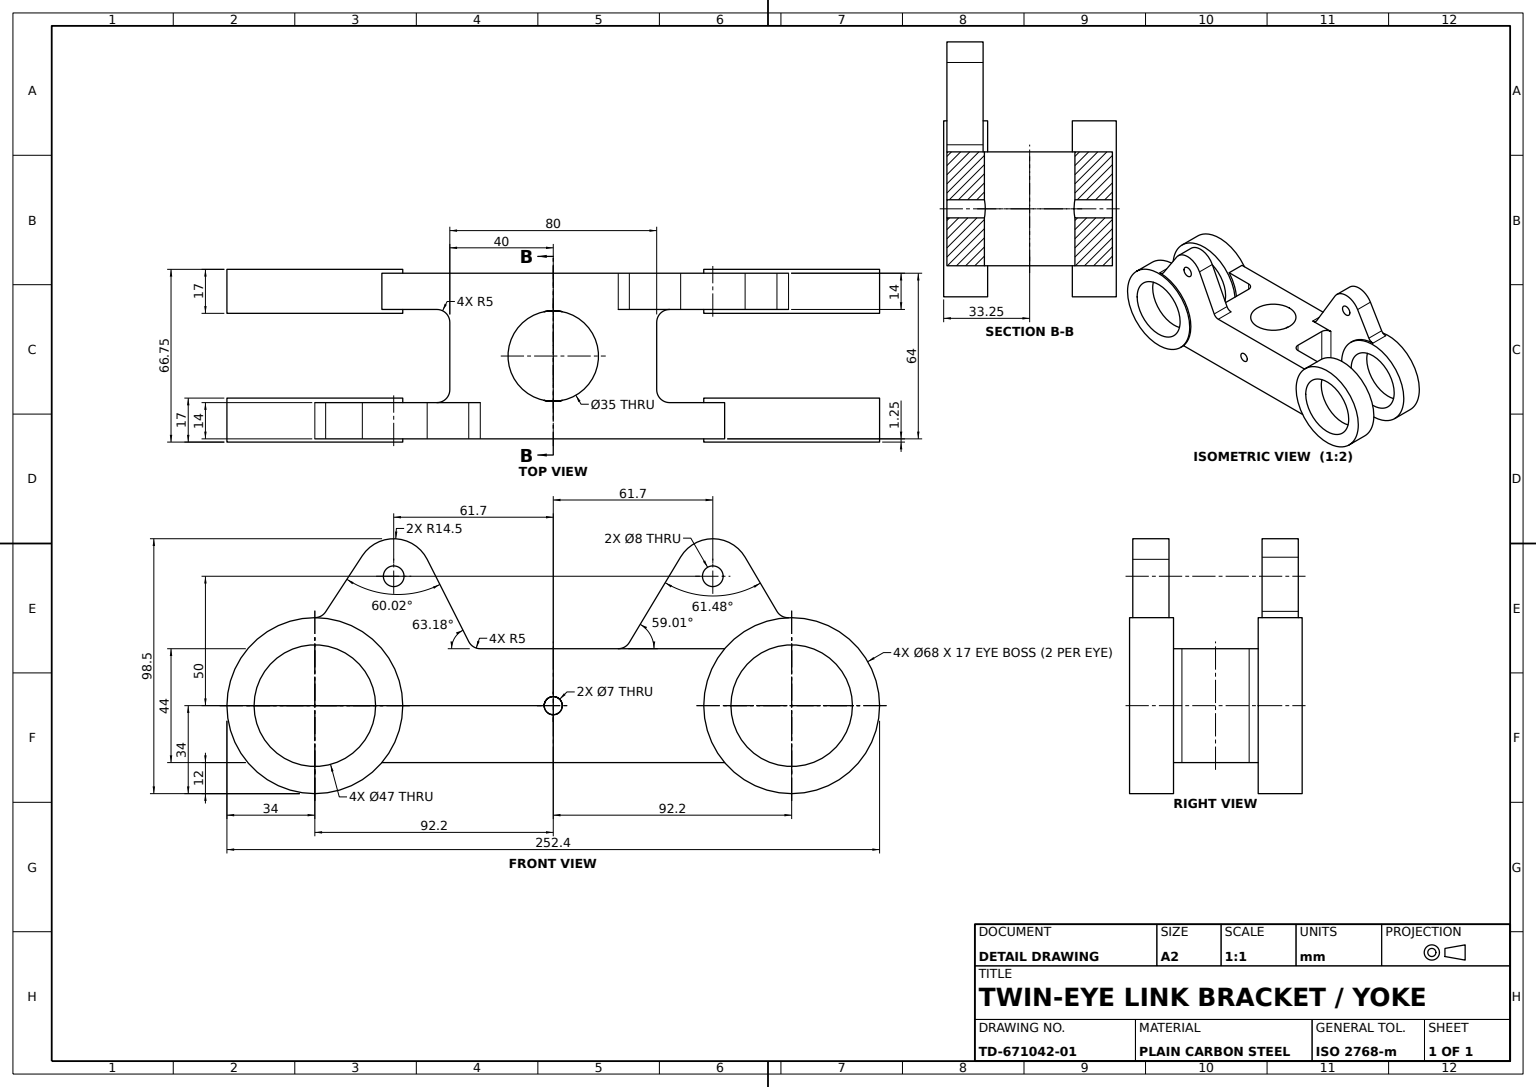
SolidWorks part; units mm, degrees
material "Plain Carbon Steel"
ref_plane "Front Plane" through (0, 0, 0) normal (0, 0, 1) x (1, 0, 0)
ref_plane "Top Plane" through (0, 0, 0) normal (0, 1, 0) x (1, 0, 0)
ref_plane "Right Plane" through (0, 0, 0) normal (1, 0, 0) x (0, 0, -1)
sketch "Center Body Sketch" plane through (0, 0, 0) normal (0, 1, 0) x (1, 0, 0)
  line L1 (-40, -32) -> (40, -32)
  line L2 (-40, -32) -> (-40, 32)
  line L3 (-40, 32) -> (40, 32)
  line L4 (40, -32) -> (40, 32)
  line L5 (-40, -32) -> (40, 32) construction
  line L6 (-40, 32) -> (40, -32) construction
  circle A0 centre (0, 0) radius 17.5
  point P0 (0, 0)
  dimension "D3" = 35
  dimension "D1" = 64
  dimension "D2" = 80
extrude "Center Body" add sketch "Center Body Sketch" along normal blind 44
sketch "Pivot Eyes Sketch" plane through (0, 0, 32) normal (0, 0, 1) x (1, 0, 0)
  line L0 (-40, 44) -> (40, 44) construction
  circle A0 centre (-92.2, 22) radius 23.5
  circle A1 centre (-92.2, 22) radius 34
  circle A2 centre (92.2, 22) radius 23.5
  circle A3 centre (92.2, 22) radius 34
  dimension "D1" = 68
  dimension "D2" = 47
  dimension "D3" = 68
  dimension "D4" = 47
  dimension "D5" = 92.2
  dimension "D6" = 92.2
  dimension "D7" = 22
  dimension "D8" = 22
extrude "Pivot Eyes Ø68xØ47" add sketch "Pivot Eyes Sketch" against normal blind 15.75 separate body
sketch "Eye Face Pads Sketch" plane through (0, 0, 32) normal (0, 0, 1) x (1, 0, 0)
  circle A0 centre (-92.2, 22) radius 23.5
  circle A1 centre (-92.2, 22) radius 34
  circle A2 centre (92.2, 22) radius 23.5
  circle A3 centre (92.2, 22) radius 34
  dimension "D1" = 68
  dimension "D2" = 47
  dimension "D3" = 68
  dimension "D4" = 47
extrude "Eye Face Pads" add sketch "Eye Face Pads Sketch" along normal blind 1.25
ref_plane "Lug Offset Plane" through (0, 0, 25) normal (0, 0, 1) x (1, 0, 0)
sketch "Mounting Lug A Sketch" plane through (0, 0, 25) normal (0, 0, 1) x (1, 0, 0)
  line L0 (40, 44) -> (67.4662, 44)
  line L1 (-40, 44) -> (-40, 0)
  line L2 (-40, 0) -> (-66.277, 0)
  line L3 (67.4662, 44) -> (67.4662, 0)
  line L4 (-73.8337, 79.9388) -> (-88.016, 58.2625)
  line L5 (-48.7603, 78.5433) -> (-32.68, 46.7437)
  line L6 (-40, 44) -> (-28.218, 44)
  line L7 (-40, 44) -> (40, 44) construction
  line L8 (67.4662, 0) -> (40, 0)
  line L9 (40, 44) -> (40, 0)
  circle A0 centre (-61.7, 72) radius 4
  arc A1 (-48.7603, 78.5433) -> (-73.8337, 79.9388) centre (-61.7, 72) ccw
  arc A4 (-66.277, 0) -> (-92.2, 56) centre (-92.2, 22) ccw
  arc A5 (-92.2, 56) -> (-88.016, 58.2625) centre (-92.2, 61) ccw
  arc A6 (-32.68, 46.7437) -> (-28.218, 44) centre (-28.218, 49) ccw
  dimension "D1" = 29
  dimension "D2" = 27.4662
  dimension "D3" = 95.6843
  dimension "D4" = 8
  dimension "D11" = 5
  dimension "D9" = 5
  dimension "D10" = 68
  dimension "D5" = 50
  dimension "D7" = 61.7
extrude "Mounting Lug A" add sketch "Mounting Lug A Sketch" along normal mid plane 14
sketch "Mounting Lug B Sketch" plane through (0, 0, -32) normal (0, 0, -1) x (-1, 0, 0)
  line L0 (40, 0) -> (40, 44) construction
  line L1 (-40, 44) -> (40, 44) construction
  line L2 (-40, 44) -> (-25.1353, 44)
  line L4 (-74.196, 79.3553) -> (-86.5074, 58.4392)
  line L5 (-49.2703, 79.4668) -> (-29.4214, 46.4252)
  line L6 (-66.277, 0) -> (-40, 0)
  line L7 (-40, 0) -> (-66.277, 0) construction
  line L8 (-40, 0) -> (-40, 44)
  circle A0 centre (-61.7, 72) radius 4
  arc A1 (-49.2703, 79.4668) -> (-74.196, 79.3553) centre (-61.7, 72) ccw
  arc A3 (-66.277, 0) -> (-90.9938, 55.9786) centre (-92.2, 22) ccw
  arc A4 (-90.9938, 55.9786) -> (-86.5074, 58.4392) centre (-90.8164, 60.9754) ccw
  arc A5 (-29.4214, 46.4252) -> (-25.1353, 44) centre (-25.1353, 49) ccw
  point P6 (40, 22)
  dimension "D1" = 29
  dimension "D2" = 8
  dimension "D7" = 5
  dimension "D5" = 34
  dimension "D8" = 38.5452
  dimension "D9" = 5
  dimension "D3" = 61.7
  dimension "D4" = 50
  dimension "D6" = 24.2704
extrude "Mounting Lug B" add sketch "Mounting Lug B Sketch" against normal blind 14
ref_plane "Offset Eye Plane" through (0, 0, -25) normal (0, 0, 1) x (1, 0, 0)
sketch "Offset Pivot Eyes Sketch" plane through (0, 0, -25) normal (0, 0, 1) x (1, 0, 0)
  circle A0 centre (92.2, 22) radius 23.5
  circle A1 centre (92.2, 22) radius 34
  circle A2 centre (-92.2, 22) radius 23.5
  circle A3 centre (-92.2, 22) radius 34
  dimension "D1" = 68
  dimension "D2" = 68
  dimension "D3" = 47
  dimension "D4" = 47
extrude "Offset Pivot Eyes" add sketch "Offset Pivot Eyes Sketch" along normal mid plane 17
sketch "Center Web Sketch" plane through (0, 0, -32) normal (0, 0, -1) x (-1, 0, 0)
  line L0 (40, 44) -> (68.2514, 44)
  line L1 (68.2514, 44) -> (68.2514, 0)
  line L2 (68.2514, 0) -> (40, 0)
  line L3 (40, 0) -> (40, 44)
  dimension "D1" = 28.2514
extrude "Center Web" add sketch "Center Web Sketch" against normal blind 14
sketch "Pin Hole Sketch" plane through (0, 0, -32) normal (0, 0, -1) x (-1, 0, 0)
  line L0 (-25.1353, 44) -> (66.277, 44) construction
  circle A0 centre (0, 22) radius 3.5
  arc A1 (66.277, 44) -> (66.277, 0) centre (92.2, 22) ccw construction
  point P7 (58.2, 22)
  dimension "D1" = 7
  dimension "D2" = 22
  dimension "D3" = 58.2
extrude "Pin Hole Ø7" cut sketch "Pin Hole Sketch" against normal blind 200
fillet "Lug A Fillets R5" radius 5 2 edges at (-40, 22, -18) (-40, 22, 18)
fillet "Lug B Fillets R5" radius 5 2 edges at (40, 22, -18) (40, 22, 18)
